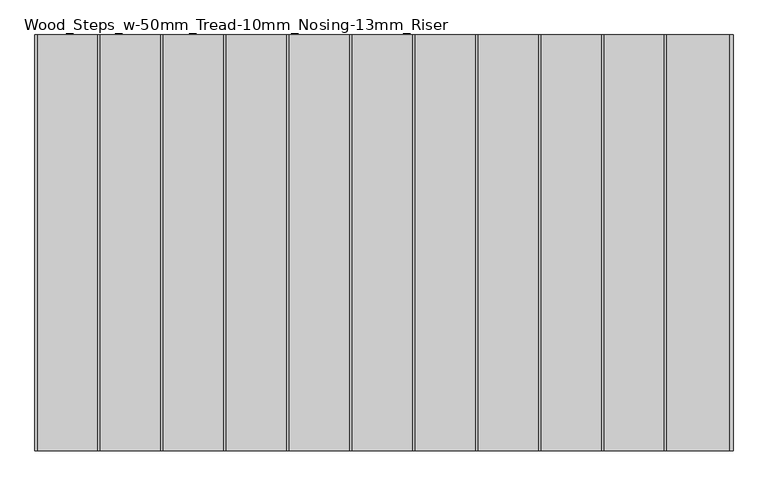
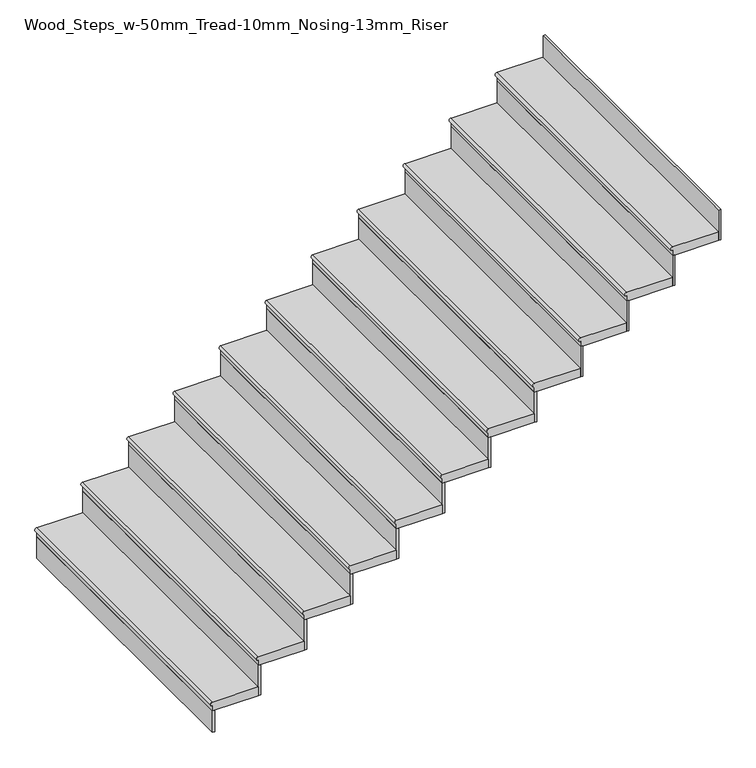
"""IFC4 building model written with IfcOpenShell, lengths in millimetres: stair flight geometry, Wood_Steps_w-50mm_Tread-10mm_Nosing-13mm_Riser."""

from ifc_helpers import new_model, si_unit, frame, origin, place, context, project, spatial, circle_curve, faceted_brep, source, transform, mapped, element, save
from ifc_brep_helpers import plane_surface, cylinder_surface, advanced_brep


def wood_steps_w_50mm_tread_10mm_nosing_13mm_riser_0f893a5b(model_context):
    return source(origin(), model_context, "Body", "SolidModel", [
        advanced_brep(
        [(-512.9988863, -6137.6352742, 153.9130435), (-512.9988863, -6137.6352742, 173.9130435), (-512.9988863, -4486.6352742, 173.9130435), (-512.9988863, -4486.6352742, 153.9130435), (-262.9988863, -4486.6352742, 173.9130435), (-262.9988863, -6137.6352742, 173.9130435), (-512.9988863, -4486.6352742, 123.9130435), (-262.9988863, -4486.6352742, 123.9130435), (-262.9988863, -6137.6352742, 123.9130435), (-512.9988863, -6137.6352742, 123.9130435)],
        [
            (0, 1, circle_curve(frame((-512.9988863, -6137.6352742, 163.9130435), z_axis=(0.0, 1.0, 0.0), x_axis=(1.0, 0.0, 0.0)), 10.0)),
            (1, 2),
            (2, 3, circle_curve(frame((-512.9988863, -4486.6352742, 163.9130435), z_axis=(0.0, -1.0, 0.0), x_axis=(1.0, 0.0, 0.0)), 10.0)),
            (3, 0),
            (4, 2),
            (1, 5),
            (5, 4),
            (6, 7),
            (7, 8),
            (8, 9),
            (9, 6),
            (4, 7),
            (6, 3),
            (9, 0),
            (8, 5),
        ],
        [
            cylinder_surface(frame((-512.9988863, -6137.6352742, 163.9130435), z_axis=(0.0, -1.0, 0.0), x_axis=(1.0, 0.0, 0.0)), 10.0),
            plane_surface(frame((-522.9988863, -4486.6352742, 173.9130435), z_axis=(0.0, 0.0, 1.0), x_axis=(-1.0, 0.0, 0.0))),
            plane_surface(frame((-522.9988863, -4486.6352742, 123.9130435), z_axis=(0.0, 0.0, -1.0), x_axis=(1.0, 0.0, 0.0))),
            plane_surface(frame((-262.9988863, -4486.6352742, 173.9130435), z_axis=(0.0, 1.0, 0.0), x_axis=(0.0, 0.0, -1.0))),
            plane_surface(frame((-512.9988863, -4486.6352742, 173.9130435), z_axis=(-1.0, 0.0, 0.0), x_axis=(0.0, 0.0, -1.0))),
            plane_surface(frame((-512.9988863, -6137.6352742, 173.9130435), z_axis=(0.0, -1.0, 0.0), x_axis=(0.0, 0.0, -1.0))),
            plane_surface(frame((-262.9988863, -6137.6352742, 173.9130435), z_axis=(1.0, 0.0, 0.0), x_axis=(0.0, 0.0, -1.0))),
        ],
        [
            (0, [[1, 2, 3, 4]]),
            (1, [[5, -2, 6, 7]]),
            (2, [[8, 9, 10, 11]]),
            (3, [[-5, 12, -8, 13, -3]]),
            (4, [[-11, 14, -4, -13]]),
            (5, [[-6, -1, -14, -10, 15]]),
            (6, [[-7, -15, -9, -12]]),
        ],
    ),
        faceted_brep([(-512.9988863, -6137.6352742, 123.9130435), (-512.9988863, -6137.6352742, 0.0), (-500.4988863, -6137.6352742, 0.0), (-500.4988863, -6137.6352742, 123.9130435), (-512.9988863, -4486.6352742, 123.9130435), (-500.4988863, -4486.6352742, 123.9130435), (-500.4988863, -4486.6352742, 0.0), (-512.9988863, -4486.6352742, 0.0)], [[[0, 1, 2, 3]], [[4, 5, 6, 7]], [[1, 0, 4, 7]], [[2, 1, 7, 6]], [[3, 2, 6, 5]], [[0, 3, 5, 4]]]),
        faceted_brep([(-262.9988863, -6137.6352742, 297.826087), (-262.9988863, -6137.6352742, 123.9130435), (-250.4988863, -6137.6352742, 123.9130435), (-250.4988863, -6137.6352742, 297.826087), (-262.9988863, -4486.6352742, 297.826087), (-250.4988863, -4486.6352742, 297.826087), (-250.4988863, -4486.6352742, 123.9130435), (-262.9988863, -4486.6352742, 123.9130435)], [[[0, 1, 2, 3]], [[4, 5, 6, 7]], [[1, 0, 4, 7]], [[2, 1, 7, 6]], [[3, 2, 6, 5]], [[0, 3, 5, 4]]]),
        advanced_brep(
        [(-12.9988863, -4486.6352742, 347.826087), (-262.9988863, -4486.6352742, 347.826087), (-262.9988863, -6137.6352742, 347.826087), (-12.9988863, -6137.6352742, 347.826087), (-262.9988863, -4486.6352742, 297.826087), (-12.9988863, -4486.6352742, 297.826087), (-12.9988863, -6137.6352742, 297.826087), (-262.9988863, -6137.6352742, 297.826087), (-262.9988863, -4486.6352742, 327.826087), (-262.9988863, -6137.6352742, 327.826087)],
        [
            (0, 1),
            (1, 2),
            (2, 3),
            (3, 0),
            (4, 5),
            (5, 6),
            (6, 7),
            (7, 4),
            (0, 5),
            (4, 8),
            (8, 1, circle_curve(frame((-262.9988863, -4486.6352742, 337.826087), z_axis=(0.0, 1.0, 0.0), x_axis=(1.0, 0.0, 0.0)), 10.0)),
            (7, 9),
            (9, 8),
            (2, 9, circle_curve(frame((-262.9988863, -6137.6352742, 337.826087), z_axis=(0.0, -1.0, 0.0), x_axis=(1.0, 0.0, 0.0)), 10.0)),
            (6, 3),
        ],
        [
            plane_surface(frame((-522.9988863, -4486.6352742, 347.826087), z_axis=(0.0, 0.0, 1.0), x_axis=(-1.0, 0.0, 0.0))),
            plane_surface(frame((-522.9988863, -4486.6352742, 297.826087), z_axis=(0.0, 0.0, -1.0), x_axis=(1.0, 0.0, 0.0))),
            plane_surface(frame((-12.9988863, -4486.6352742, 347.826087), z_axis=(0.0, 1.0, 0.0), x_axis=(0.0, 0.0, -1.0))),
            plane_surface(frame((-262.9988863, -4486.6352742, 347.826087), z_axis=(-1.0, 0.0, 0.0), x_axis=(0.0, 0.0, -1.0))),
            plane_surface(frame((-262.9988863, -6137.6352742, 347.826087), z_axis=(0.0, -1.0, 0.0), x_axis=(0.0, 0.0, -1.0))),
            plane_surface(frame((-12.9988863, -6137.6352742, 347.826087), z_axis=(1.0, 0.0, 0.0), x_axis=(0.0, 0.0, -1.0))),
            cylinder_surface(frame((-262.9988863, -6137.6352742, 337.826087), z_axis=(0.0, -1.0, 0.0), x_axis=(1.0, 0.0, 0.0)), 10.0),
        ],
        [
            (0, [[1, 2, 3, 4]]),
            (1, [[5, 6, 7, 8]]),
            (2, [[-1, 9, -5, 10, 11]]),
            (3, [[-8, 12, 13, -10]]),
            (4, [[-3, 14, -12, -7, 15]]),
            (5, [[-4, -15, -6, -9]]),
            (6, [[-14, -2, -11, -13]]),
        ],
    ),
        faceted_brep([(-12.9988863, -6137.6352742, 471.7391304), (-12.9988863, -6137.6352742, 297.826087), (-0.4988863, -6137.6352742, 297.826087), (-0.4988863, -6137.6352742, 471.7391304), (-12.9988863, -4486.6352742, 471.7391304), (-0.4988863, -4486.6352742, 471.7391304), (-0.4988863, -4486.6352742, 297.826087), (-12.9988863, -4486.6352742, 297.826087)], [[[0, 1, 2, 3]], [[4, 5, 6, 7]], [[1, 0, 4, 7]], [[2, 1, 7, 6]], [[3, 2, 6, 5]], [[0, 3, 5, 4]]]),
        advanced_brep(
        [(237.0011137, -4486.6352742, 521.7391304), (-12.9988863, -4486.6352742, 521.7391304), (-12.9988863, -6137.6352742, 521.7391304), (237.0011137, -6137.6352742, 521.7391304), (-12.9988863, -4486.6352742, 471.7391304), (237.0011137, -4486.6352742, 471.7391304), (237.0011137, -6137.6352742, 471.7391304), (-12.9988863, -6137.6352742, 471.7391304), (-12.9988863, -4486.6352742, 501.7391304), (-12.9988863, -6137.6352742, 501.7391304)],
        [
            (0, 1),
            (1, 2),
            (2, 3),
            (3, 0),
            (4, 5),
            (5, 6),
            (6, 7),
            (7, 4),
            (0, 5),
            (4, 8),
            (8, 1, circle_curve(frame((-12.9988863, -4486.6352742, 511.7391304), z_axis=(0.0, 1.0, 0.0), x_axis=(1.0, 0.0, 0.0)), 10.0)),
            (7, 9),
            (9, 8),
            (2, 9, circle_curve(frame((-12.9988863, -6137.6352742, 511.7391304), z_axis=(0.0, -1.0, 0.0), x_axis=(1.0, 0.0, 0.0)), 10.0)),
            (6, 3),
        ],
        [
            plane_surface(frame((-272.9988863, -4486.6352742, 521.7391304), z_axis=(0.0, 0.0, 1.0), x_axis=(-1.0, 0.0, 0.0))),
            plane_surface(frame((-272.9988863, -4486.6352742, 471.7391304), z_axis=(0.0, 0.0, -1.0), x_axis=(1.0, 0.0, 0.0))),
            plane_surface(frame((237.0011137, -4486.6352742, 521.7391304), z_axis=(0.0, 1.0, 0.0), x_axis=(0.0, 0.0, -1.0))),
            plane_surface(frame((-12.9988863, -4486.6352742, 521.7391304), z_axis=(-1.0, 0.0, 0.0), x_axis=(0.0, 0.0, -1.0))),
            plane_surface(frame((-12.9988863, -6137.6352742, 521.7391304), z_axis=(0.0, -1.0, 0.0), x_axis=(0.0, 0.0, -1.0))),
            plane_surface(frame((237.0011137, -6137.6352742, 521.7391304), z_axis=(1.0, 0.0, 0.0), x_axis=(0.0, 0.0, -1.0))),
            cylinder_surface(frame((-12.9988863, -6137.6352742, 511.7391304), z_axis=(0.0, -1.0, 0.0), x_axis=(1.0, 0.0, 0.0)), 10.0),
        ],
        [
            (0, [[1, 2, 3, 4]]),
            (1, [[5, 6, 7, 8]]),
            (2, [[-1, 9, -5, 10, 11]]),
            (3, [[-8, 12, 13, -10]]),
            (4, [[-3, 14, -12, -7, 15]]),
            (5, [[-4, -15, -6, -9]]),
            (6, [[-14, -2, -11, -13]]),
        ],
    ),
        faceted_brep([(237.0011137, -6137.6352742, 645.6521739), (237.0011137, -6137.6352742, 471.7391304), (249.5011137, -6137.6352742, 471.7391304), (249.5011137, -6137.6352742, 645.6521739), (237.0011137, -4486.6352742, 645.6521739), (249.5011137, -4486.6352742, 645.6521739), (249.5011137, -4486.6352742, 471.7391304), (237.0011137, -4486.6352742, 471.7391304)], [[[0, 1, 2, 3]], [[4, 5, 6, 7]], [[1, 0, 4, 7]], [[2, 1, 7, 6]], [[3, 2, 6, 5]], [[0, 3, 5, 4]]]),
        advanced_brep(
        [(487.0011137, -4486.6352742, 695.6521739), (237.0011137, -4486.6352742, 695.6521739), (237.0011137, -6137.6352742, 695.6521739), (487.0011137, -6137.6352742, 695.6521739), (237.0011137, -4486.6352742, 645.6521739), (487.0011137, -4486.6352742, 645.6521739), (487.0011137, -6137.6352742, 645.6521739), (237.0011137, -6137.6352742, 645.6521739), (237.0011137, -4486.6352742, 675.6521739), (237.0011137, -6137.6352742, 675.6521739)],
        [
            (0, 1),
            (1, 2),
            (2, 3),
            (3, 0),
            (4, 5),
            (5, 6),
            (6, 7),
            (7, 4),
            (0, 5),
            (4, 8),
            (8, 1, circle_curve(frame((237.0011137, -4486.6352742, 685.6521739), z_axis=(0.0, 1.0, 0.0), x_axis=(1.0, 0.0, 0.0)), 10.0)),
            (7, 9),
            (9, 8),
            (2, 9, circle_curve(frame((237.0011137, -6137.6352742, 685.6521739), z_axis=(0.0, -1.0, 0.0), x_axis=(1.0, 0.0, 0.0)), 10.0)),
            (6, 3),
        ],
        [
            plane_surface(frame((-22.9988863, -4486.6352742, 695.6521739), z_axis=(0.0, 0.0, 1.0), x_axis=(-1.0, 0.0, 0.0))),
            plane_surface(frame((-22.9988863, -4486.6352742, 645.6521739), z_axis=(0.0, 0.0, -1.0), x_axis=(1.0, 0.0, 0.0))),
            plane_surface(frame((487.0011137, -4486.6352742, 695.6521739), z_axis=(0.0, 1.0, 0.0), x_axis=(0.0, 0.0, -1.0))),
            plane_surface(frame((237.0011137, -4486.6352742, 695.6521739), z_axis=(-1.0, 0.0, 0.0), x_axis=(0.0, 0.0, -1.0))),
            plane_surface(frame((237.0011137, -6137.6352742, 695.6521739), z_axis=(0.0, -1.0, 0.0), x_axis=(0.0, 0.0, -1.0))),
            plane_surface(frame((487.0011137, -6137.6352742, 695.6521739), z_axis=(1.0, 0.0, 0.0), x_axis=(0.0, 0.0, -1.0))),
            cylinder_surface(frame((237.0011137, -6137.6352742, 685.6521739), z_axis=(0.0, -1.0, 0.0), x_axis=(1.0, 0.0, 0.0)), 10.0),
        ],
        [
            (0, [[1, 2, 3, 4]]),
            (1, [[5, 6, 7, 8]]),
            (2, [[-1, 9, -5, 10, 11]]),
            (3, [[-8, 12, 13, -10]]),
            (4, [[-3, 14, -12, -7, 15]]),
            (5, [[-4, -15, -6, -9]]),
            (6, [[-14, -2, -11, -13]]),
        ],
    ),
        faceted_brep([(487.0011137, -6137.6352742, 819.5652174), (487.0011137, -6137.6352742, 645.6521739), (499.5011137, -6137.6352742, 645.6521739), (499.5011137, -6137.6352742, 819.5652174), (487.0011137, -4486.6352742, 819.5652174), (499.5011137, -4486.6352742, 819.5652174), (499.5011137, -4486.6352742, 645.6521739), (487.0011137, -4486.6352742, 645.6521739)], [[[0, 1, 2, 3]], [[4, 5, 6, 7]], [[1, 0, 4, 7]], [[2, 1, 7, 6]], [[3, 2, 6, 5]], [[0, 3, 5, 4]]]),
        advanced_brep(
        [(737.0011137, -4486.6352742, 869.5652174), (487.0011137, -4486.6352742, 869.5652174), (487.0011137, -6137.6352742, 869.5652174), (737.0011137, -6137.6352742, 869.5652174), (487.0011137, -4486.6352742, 819.5652174), (737.0011137, -4486.6352742, 819.5652174), (737.0011137, -6137.6352742, 819.5652174), (487.0011137, -6137.6352742, 819.5652174), (487.0011137, -4486.6352742, 849.5652174), (487.0011137, -6137.6352742, 849.5652174)],
        [
            (0, 1),
            (1, 2),
            (2, 3),
            (3, 0),
            (4, 5),
            (5, 6),
            (6, 7),
            (7, 4),
            (0, 5),
            (4, 8),
            (8, 1, circle_curve(frame((487.0011137, -4486.6352742, 859.5652174), z_axis=(0.0, 1.0, 0.0), x_axis=(1.0, 0.0, 0.0)), 10.0)),
            (7, 9),
            (9, 8),
            (2, 9, circle_curve(frame((487.0011137, -6137.6352742, 859.5652174), z_axis=(0.0, -1.0, 0.0), x_axis=(1.0, 0.0, 0.0)), 10.0)),
            (6, 3),
        ],
        [
            plane_surface(frame((227.0011137, -4486.6352742, 869.5652174), z_axis=(0.0, 0.0, 1.0), x_axis=(-1.0, 0.0, 0.0))),
            plane_surface(frame((227.0011137, -4486.6352742, 819.5652174), z_axis=(0.0, 0.0, -1.0), x_axis=(1.0, 0.0, 0.0))),
            plane_surface(frame((737.0011137, -4486.6352742, 869.5652174), z_axis=(0.0, 1.0, 0.0), x_axis=(0.0, 0.0, -1.0))),
            plane_surface(frame((487.0011137, -4486.6352742, 869.5652174), z_axis=(-1.0, 0.0, 0.0), x_axis=(0.0, 0.0, -1.0))),
            plane_surface(frame((487.0011137, -6137.6352742, 869.5652174), z_axis=(0.0, -1.0, 0.0), x_axis=(0.0, 0.0, -1.0))),
            plane_surface(frame((737.0011137, -6137.6352742, 869.5652174), z_axis=(1.0, 0.0, 0.0), x_axis=(0.0, 0.0, -1.0))),
            cylinder_surface(frame((487.0011137, -6137.6352742, 859.5652174), z_axis=(0.0, -1.0, 0.0), x_axis=(1.0, 0.0, 0.0)), 10.0),
        ],
        [
            (0, [[1, 2, 3, 4]]),
            (1, [[5, 6, 7, 8]]),
            (2, [[-1, 9, -5, 10, 11]]),
            (3, [[-8, 12, 13, -10]]),
            (4, [[-3, 14, -12, -7, 15]]),
            (5, [[-4, -15, -6, -9]]),
            (6, [[-14, -2, -11, -13]]),
        ],
    ),
        faceted_brep([(737.0011137, -6137.6352742, 993.4782609), (737.0011137, -6137.6352742, 819.5652174), (749.5011137, -6137.6352742, 819.5652174), (749.5011137, -6137.6352742, 993.4782609), (737.0011137, -4486.6352742, 993.4782609), (749.5011137, -4486.6352742, 993.4782609), (749.5011137, -4486.6352742, 819.5652174), (737.0011137, -4486.6352742, 819.5652174)], [[[0, 1, 2, 3]], [[4, 5, 6, 7]], [[1, 0, 4, 7]], [[2, 1, 7, 6]], [[3, 2, 6, 5]], [[0, 3, 5, 4]]]),
        advanced_brep(
        [(987.0011137, -4486.6352742, 1043.4782609), (737.0011137, -4486.6352742, 1043.4782609), (737.0011137, -6137.6352742, 1043.4782609), (987.0011137, -6137.6352742, 1043.4782609), (737.0011137, -4486.6352742, 993.4782609), (987.0011137, -4486.6352742, 993.4782609), (987.0011137, -6137.6352742, 993.4782609), (737.0011137, -6137.6352742, 993.4782609), (737.0011137, -4486.6352742, 1023.4782609), (737.0011137, -6137.6352742, 1023.4782609)],
        [
            (0, 1),
            (1, 2),
            (2, 3),
            (3, 0),
            (4, 5),
            (5, 6),
            (6, 7),
            (7, 4),
            (0, 5),
            (4, 8),
            (8, 1, circle_curve(frame((737.0011137, -4486.6352742, 1033.4782609), z_axis=(0.0, 1.0, 0.0), x_axis=(1.0, 0.0, 0.0)), 10.0)),
            (7, 9),
            (9, 8),
            (2, 9, circle_curve(frame((737.0011137, -6137.6352742, 1033.4782609), z_axis=(0.0, -1.0, 0.0), x_axis=(1.0, 0.0, 0.0)), 10.0)),
            (6, 3),
        ],
        [
            plane_surface(frame((477.0011137, -4486.6352742, 1043.4782609), z_axis=(0.0, 0.0, 1.0), x_axis=(-1.0, 0.0, 0.0))),
            plane_surface(frame((477.0011137, -4486.6352742, 993.4782609), z_axis=(0.0, 0.0, -1.0), x_axis=(1.0, 0.0, 0.0))),
            plane_surface(frame((987.0011137, -4486.6352742, 1043.4782609), z_axis=(0.0, 1.0, 0.0), x_axis=(0.0, 0.0, -1.0))),
            plane_surface(frame((737.0011137, -4486.6352742, 1043.4782609), z_axis=(-1.0, 0.0, 0.0), x_axis=(0.0, 0.0, -1.0))),
            plane_surface(frame((737.0011137, -6137.6352742, 1043.4782609), z_axis=(0.0, -1.0, 0.0), x_axis=(0.0, 0.0, -1.0))),
            plane_surface(frame((987.0011137, -6137.6352742, 1043.4782609), z_axis=(1.0, 0.0, 0.0), x_axis=(0.0, 0.0, -1.0))),
            cylinder_surface(frame((737.0011137, -6137.6352742, 1033.4782609), z_axis=(0.0, -1.0, 0.0), x_axis=(1.0, 0.0, 0.0)), 10.0),
        ],
        [
            (0, [[1, 2, 3, 4]]),
            (1, [[5, 6, 7, 8]]),
            (2, [[-1, 9, -5, 10, 11]]),
            (3, [[-8, 12, 13, -10]]),
            (4, [[-3, 14, -12, -7, 15]]),
            (5, [[-4, -15, -6, -9]]),
            (6, [[-14, -2, -11, -13]]),
        ],
    ),
        faceted_brep([(987.0011137, -6137.6352742, 1167.3913043), (987.0011137, -6137.6352742, 993.4782609), (999.5011137, -6137.6352742, 993.4782609), (999.5011137, -6137.6352742, 1167.3913043), (987.0011137, -4486.6352742, 1167.3913043), (999.5011137, -4486.6352742, 1167.3913043), (999.5011137, -4486.6352742, 993.4782609), (987.0011137, -4486.6352742, 993.4782609)], [[[0, 1, 2, 3]], [[4, 5, 6, 7]], [[1, 0, 4, 7]], [[2, 1, 7, 6]], [[3, 2, 6, 5]], [[0, 3, 5, 4]]]),
        advanced_brep(
        [(1237.0011137, -4486.6352742, 1217.3913043), (987.0011137, -4486.6352742, 1217.3913043), (987.0011137, -6137.6352742, 1217.3913043), (1237.0011137, -6137.6352742, 1217.3913043), (987.0011137, -4486.6352742, 1167.3913043), (1237.0011137, -4486.6352742, 1167.3913043), (1237.0011137, -6137.6352742, 1167.3913043), (987.0011137, -6137.6352742, 1167.3913043), (987.0011137, -4486.6352742, 1197.3913043), (987.0011137, -6137.6352742, 1197.3913043)],
        [
            (0, 1),
            (1, 2),
            (2, 3),
            (3, 0),
            (4, 5),
            (5, 6),
            (6, 7),
            (7, 4),
            (0, 5),
            (4, 8),
            (8, 1, circle_curve(frame((987.0011137, -4486.6352742, 1207.3913043), z_axis=(0.0, 1.0, 0.0), x_axis=(1.0, 0.0, 0.0)), 10.0)),
            (7, 9),
            (9, 8),
            (2, 9, circle_curve(frame((987.0011137, -6137.6352742, 1207.3913043), z_axis=(0.0, -1.0, 0.0), x_axis=(1.0, 0.0, 0.0)), 10.0)),
            (6, 3),
        ],
        [
            plane_surface(frame((727.0011137, -4486.6352742, 1217.3913043), z_axis=(0.0, 0.0, 1.0), x_axis=(-1.0, 0.0, 0.0))),
            plane_surface(frame((727.0011137, -4486.6352742, 1167.3913043), z_axis=(0.0, 0.0, -1.0), x_axis=(1.0, 0.0, 0.0))),
            plane_surface(frame((1237.0011137, -4486.6352742, 1217.3913043), z_axis=(0.0, 1.0, 0.0), x_axis=(0.0, 0.0, -1.0))),
            plane_surface(frame((987.0011137, -4486.6352742, 1217.3913043), z_axis=(-1.0, 0.0, 0.0), x_axis=(0.0, 0.0, -1.0))),
            plane_surface(frame((987.0011137, -6137.6352742, 1217.3913043), z_axis=(0.0, -1.0, 0.0), x_axis=(0.0, 0.0, -1.0))),
            plane_surface(frame((1237.0011137, -6137.6352742, 1217.3913043), z_axis=(1.0, 0.0, 0.0), x_axis=(0.0, 0.0, -1.0))),
            cylinder_surface(frame((987.0011137, -6137.6352742, 1207.3913043), z_axis=(0.0, -1.0, 0.0), x_axis=(1.0, 0.0, 0.0)), 10.0),
        ],
        [
            (0, [[1, 2, 3, 4]]),
            (1, [[5, 6, 7, 8]]),
            (2, [[-1, 9, -5, 10, 11]]),
            (3, [[-8, 12, 13, -10]]),
            (4, [[-3, 14, -12, -7, 15]]),
            (5, [[-4, -15, -6, -9]]),
            (6, [[-14, -2, -11, -13]]),
        ],
    ),
        faceted_brep([(1237.0011137, -6137.6352742, 1341.3043478), (1237.0011137, -6137.6352742, 1167.3913043), (1249.5011137, -6137.6352742, 1167.3913043), (1249.5011137, -6137.6352742, 1341.3043478), (1237.0011137, -4486.6352742, 1341.3043478), (1249.5011137, -4486.6352742, 1341.3043478), (1249.5011137, -4486.6352742, 1167.3913043), (1237.0011137, -4486.6352742, 1167.3913043)], [[[0, 1, 2, 3]], [[4, 5, 6, 7]], [[1, 0, 4, 7]], [[2, 1, 7, 6]], [[3, 2, 6, 5]], [[0, 3, 5, 4]]]),
        advanced_brep(
        [(1487.0011137, -4486.6352742, 1391.3043478), (1237.0011137, -4486.6352742, 1391.3043478), (1237.0011137, -6137.6352742, 1391.3043478), (1487.0011137, -6137.6352742, 1391.3043478), (1237.0011137, -4486.6352742, 1341.3043478), (1487.0011137, -4486.6352742, 1341.3043478), (1487.0011137, -6137.6352742, 1341.3043478), (1237.0011137, -6137.6352742, 1341.3043478), (1237.0011137, -4486.6352742, 1371.3043478), (1237.0011137, -6137.6352742, 1371.3043478)],
        [
            (0, 1),
            (1, 2),
            (2, 3),
            (3, 0),
            (4, 5),
            (5, 6),
            (6, 7),
            (7, 4),
            (0, 5),
            (4, 8),
            (8, 1, circle_curve(frame((1237.0011137, -4486.6352742, 1381.3043478), z_axis=(0.0, 1.0, 0.0), x_axis=(1.0, 0.0, 0.0)), 10.0)),
            (7, 9),
            (9, 8),
            (2, 9, circle_curve(frame((1237.0011137, -6137.6352742, 1381.3043478), z_axis=(0.0, -1.0, 0.0), x_axis=(1.0, 0.0, 0.0)), 10.0)),
            (6, 3),
        ],
        [
            plane_surface(frame((977.0011137, -4486.6352742, 1391.3043478), z_axis=(0.0, 0.0, 1.0), x_axis=(-1.0, 0.0, 0.0))),
            plane_surface(frame((977.0011137, -4486.6352742, 1341.3043478), z_axis=(0.0, 0.0, -1.0), x_axis=(1.0, 0.0, 0.0))),
            plane_surface(frame((1487.0011137, -4486.6352742, 1391.3043478), z_axis=(0.0, 1.0, 0.0), x_axis=(0.0, 0.0, -1.0))),
            plane_surface(frame((1237.0011137, -4486.6352742, 1391.3043478), z_axis=(-1.0, 0.0, 0.0), x_axis=(0.0, 0.0, -1.0))),
            plane_surface(frame((1237.0011137, -6137.6352742, 1391.3043478), z_axis=(0.0, -1.0, 0.0), x_axis=(0.0, 0.0, -1.0))),
            plane_surface(frame((1487.0011137, -6137.6352742, 1391.3043478), z_axis=(1.0, 0.0, 0.0), x_axis=(0.0, 0.0, -1.0))),
            cylinder_surface(frame((1237.0011137, -6137.6352742, 1381.3043478), z_axis=(0.0, -1.0, 0.0), x_axis=(1.0, 0.0, 0.0)), 10.0),
        ],
        [
            (0, [[1, 2, 3, 4]]),
            (1, [[5, 6, 7, 8]]),
            (2, [[-1, 9, -5, 10, 11]]),
            (3, [[-8, 12, 13, -10]]),
            (4, [[-3, 14, -12, -7, 15]]),
            (5, [[-4, -15, -6, -9]]),
            (6, [[-14, -2, -11, -13]]),
        ],
    ),
        faceted_brep([(1487.0011137, -6137.6352742, 1515.2173913), (1487.0011137, -6137.6352742, 1341.3043478), (1499.5011137, -6137.6352742, 1341.3043478), (1499.5011137, -6137.6352742, 1515.2173913), (1487.0011137, -4486.6352742, 1515.2173913), (1499.5011137, -4486.6352742, 1515.2173913), (1499.5011137, -4486.6352742, 1341.3043478), (1487.0011137, -4486.6352742, 1341.3043478)], [[[0, 1, 2, 3]], [[4, 5, 6, 7]], [[1, 0, 4, 7]], [[2, 1, 7, 6]], [[3, 2, 6, 5]], [[0, 3, 5, 4]]]),
        advanced_brep(
        [(1737.0011137, -4486.6352742, 1565.2173913), (1487.0011137, -4486.6352742, 1565.2173913), (1487.0011137, -6137.6352742, 1565.2173913), (1737.0011137, -6137.6352742, 1565.2173913), (1487.0011137, -4486.6352742, 1515.2173913), (1737.0011137, -4486.6352742, 1515.2173913), (1737.0011137, -6137.6352742, 1515.2173913), (1487.0011137, -6137.6352742, 1515.2173913), (1487.0011137, -4486.6352742, 1545.2173913), (1487.0011137, -6137.6352742, 1545.2173913)],
        [
            (0, 1),
            (1, 2),
            (2, 3),
            (3, 0),
            (4, 5),
            (5, 6),
            (6, 7),
            (7, 4),
            (0, 5),
            (4, 8),
            (8, 1, circle_curve(frame((1487.0011137, -4486.6352742, 1555.2173913), z_axis=(0.0, 1.0, 0.0), x_axis=(1.0, 0.0, 0.0)), 10.0)),
            (7, 9),
            (9, 8),
            (2, 9, circle_curve(frame((1487.0011137, -6137.6352742, 1555.2173913), z_axis=(0.0, -1.0, 0.0), x_axis=(1.0, 0.0, 0.0)), 10.0)),
            (6, 3),
        ],
        [
            plane_surface(frame((1227.0011137, -4486.6352742, 1565.2173913), z_axis=(0.0, 0.0, 1.0), x_axis=(-1.0, 0.0, 0.0))),
            plane_surface(frame((1227.0011137, -4486.6352742, 1515.2173913), z_axis=(0.0, 0.0, -1.0), x_axis=(1.0, 0.0, 0.0))),
            plane_surface(frame((1737.0011137, -4486.6352742, 1565.2173913), z_axis=(0.0, 1.0, 0.0), x_axis=(0.0, 0.0, -1.0))),
            plane_surface(frame((1487.0011137, -4486.6352742, 1565.2173913), z_axis=(-1.0, 0.0, 0.0), x_axis=(0.0, 0.0, -1.0))),
            plane_surface(frame((1487.0011137, -6137.6352742, 1565.2173913), z_axis=(0.0, -1.0, 0.0), x_axis=(0.0, 0.0, -1.0))),
            plane_surface(frame((1737.0011137, -6137.6352742, 1565.2173913), z_axis=(1.0, 0.0, 0.0), x_axis=(0.0, 0.0, -1.0))),
            cylinder_surface(frame((1487.0011137, -6137.6352742, 1555.2173913), z_axis=(0.0, -1.0, 0.0), x_axis=(1.0, 0.0, 0.0)), 10.0),
        ],
        [
            (0, [[1, 2, 3, 4]]),
            (1, [[5, 6, 7, 8]]),
            (2, [[-1, 9, -5, 10, 11]]),
            (3, [[-8, 12, 13, -10]]),
            (4, [[-3, 14, -12, -7, 15]]),
            (5, [[-4, -15, -6, -9]]),
            (6, [[-14, -2, -11, -13]]),
        ],
    ),
        faceted_brep([(1737.0011137, -6137.6352742, 1689.1304348), (1737.0011137, -6137.6352742, 1515.2173913), (1749.5011137, -6137.6352742, 1515.2173913), (1749.5011137, -6137.6352742, 1689.1304348), (1737.0011137, -4486.6352742, 1689.1304348), (1749.5011137, -4486.6352742, 1689.1304348), (1749.5011137, -4486.6352742, 1515.2173913), (1737.0011137, -4486.6352742, 1515.2173913)], [[[0, 1, 2, 3]], [[4, 5, 6, 7]], [[1, 0, 4, 7]], [[2, 1, 7, 6]], [[3, 2, 6, 5]], [[0, 3, 5, 4]]]),
        advanced_brep(
        [(1987.0011137, -4486.6352742, 1739.1304348), (1737.0011137, -4486.6352742, 1739.1304348), (1737.0011137, -6137.6352742, 1739.1304348), (1987.0011137, -6137.6352742, 1739.1304348), (1737.0011137, -4486.6352742, 1689.1304348), (1987.0011137, -4486.6352742, 1689.1304348), (1987.0011137, -6137.6352742, 1689.1304348), (1737.0011137, -6137.6352742, 1689.1304348), (1737.0011137, -4486.6352742, 1719.1304348), (1737.0011137, -6137.6352742, 1719.1304348)],
        [
            (0, 1),
            (1, 2),
            (2, 3),
            (3, 0),
            (4, 5),
            (5, 6),
            (6, 7),
            (7, 4),
            (0, 5),
            (4, 8),
            (8, 1, circle_curve(frame((1737.0011137, -4486.6352742, 1729.1304348), z_axis=(0.0, 1.0, 0.0), x_axis=(1.0, 0.0, 0.0)), 10.0)),
            (7, 9),
            (9, 8),
            (2, 9, circle_curve(frame((1737.0011137, -6137.6352742, 1729.1304348), z_axis=(0.0, -1.0, 0.0), x_axis=(1.0, 0.0, 0.0)), 10.0)),
            (6, 3),
        ],
        [
            plane_surface(frame((1477.0011137, -4486.6352742, 1739.1304348), z_axis=(0.0, 0.0, 1.0), x_axis=(-1.0, 0.0, 0.0))),
            plane_surface(frame((1477.0011137, -4486.6352742, 1689.1304348), z_axis=(0.0, 0.0, -1.0), x_axis=(1.0, 0.0, 0.0))),
            plane_surface(frame((1987.0011137, -4486.6352742, 1739.1304348), z_axis=(0.0, 1.0, 0.0), x_axis=(0.0, 0.0, -1.0))),
            plane_surface(frame((1737.0011137, -4486.6352742, 1739.1304348), z_axis=(-1.0, 0.0, 0.0), x_axis=(0.0, 0.0, -1.0))),
            plane_surface(frame((1737.0011137, -6137.6352742, 1739.1304348), z_axis=(0.0, -1.0, 0.0), x_axis=(0.0, 0.0, -1.0))),
            plane_surface(frame((1987.0011137, -6137.6352742, 1739.1304348), z_axis=(1.0, 0.0, 0.0), x_axis=(0.0, 0.0, -1.0))),
            cylinder_surface(frame((1737.0011137, -6137.6352742, 1729.1304348), z_axis=(0.0, -1.0, 0.0), x_axis=(1.0, 0.0, 0.0)), 10.0),
        ],
        [
            (0, [[1, 2, 3, 4]]),
            (1, [[5, 6, 7, 8]]),
            (2, [[-1, 9, -5, 10, 11]]),
            (3, [[-8, 12, 13, -10]]),
            (4, [[-3, 14, -12, -7, 15]]),
            (5, [[-4, -15, -6, -9]]),
            (6, [[-14, -2, -11, -13]]),
        ],
    ),
        faceted_brep([(2237.0011137, -6137.6352742, 2036.9565217), (2237.0011137, -6137.6352742, 1863.0434783), (2249.5011137, -6137.6352742, 1863.0434783), (2249.5011137, -6137.6352742, 2036.9565217), (2237.0011137, -4486.6352742, 2036.9565217), (2249.5011137, -4486.6352742, 2036.9565217), (2249.5011137, -4486.6352742, 1863.0434783), (2237.0011137, -4486.6352742, 1863.0434783)], [[[0, 1, 2, 3]], [[4, 5, 6, 7]], [[1, 0, 4, 7]], [[2, 1, 7, 6]], [[3, 2, 6, 5]], [[0, 3, 5, 4]]]),
        faceted_brep([(1987.0011137, -6137.6352742, 1863.0434783), (1987.0011137, -6137.6352742, 1689.1304348), (1999.5011137, -6137.6352742, 1689.1304348), (1999.5011137, -6137.6352742, 1863.0434783), (1987.0011137, -4486.6352742, 1863.0434783), (1999.5011137, -4486.6352742, 1863.0434783), (1999.5011137, -4486.6352742, 1689.1304348), (1987.0011137, -4486.6352742, 1689.1304348)], [[[0, 1, 2, 3]], [[4, 5, 6, 7]], [[1, 0, 4, 7]], [[2, 1, 7, 6]], [[3, 2, 6, 5]], [[0, 3, 5, 4]]]),
        advanced_brep(
        [(2237.0011137, -4486.6352742, 1913.0434783), (2227.0011137, -4486.6352742, 1913.0434783), (1987.0011137, -4486.6352742, 1913.0434783), (1987.0011137, -6137.6352742, 1913.0434783), (2237.0011137, -6137.6352742, 1913.0434783), (2227.0011137, -4486.6352742, 1863.0434783), (2237.0011137, -4486.6352742, 1863.0434783), (2237.0011137, -6137.6352742, 1863.0434783), (1987.0011137, -6137.6352742, 1863.0434783), (1987.0011137, -4486.6352742, 1863.0434783), (1987.0011137, -4486.6352742, 1893.0434783), (1987.0011137, -6137.6352742, 1893.0434783)],
        [
            (0, 1),
            (1, 2),
            (2, 3),
            (3, 4),
            (4, 0),
            (5, 6),
            (6, 7),
            (7, 8),
            (8, 9),
            (9, 5),
            (0, 6),
            (5, 1),
            (9, 10),
            (10, 2, circle_curve(frame((1987.0011137, -4486.6352742, 1903.0434783), z_axis=(0.0, 1.0, 0.0), x_axis=(1.0, 0.0, 0.0)), 10.0)),
            (8, 11),
            (11, 10),
            (3, 11, circle_curve(frame((1987.0011137, -6137.6352742, 1903.0434783), z_axis=(0.0, -1.0, 0.0), x_axis=(1.0, 0.0, 0.0)), 10.0)),
            (7, 4),
        ],
        [
            plane_surface(frame((2227.0011137, -4486.6352742, 1913.0434783), z_axis=(0.0, 0.0, 1.0), x_axis=(-1.0, 0.0, 0.0))),
            plane_surface(frame((2227.0011137, -4486.6352742, 1863.0434783), z_axis=(0.0, 0.0, -1.0), x_axis=(1.0, 0.0, 0.0))),
            plane_surface(frame((2237.0011137, -4486.6352742, 1913.0434783), z_axis=(0.0, 1.0, 0.0), x_axis=(0.0, 0.0, -1.0))),
            plane_surface(frame((2227.0011137, -4486.6352742, 1913.0434783), z_axis=(0.0, 1.0, 0.0), x_axis=(0.0, 0.0, -1.0))),
            plane_surface(frame((1987.0011137, -4486.6352742, 1913.0434783), z_axis=(-1.0, 0.0, 0.0), x_axis=(0.0, 0.0, -1.0))),
            plane_surface(frame((1987.0011137, -6137.6352742, 1913.0434783), z_axis=(0.0, -1.0, 0.0), x_axis=(0.0, 0.0, -1.0))),
            plane_surface(frame((2237.0011137, -6137.6352742, 1913.0434783), z_axis=(1.0, 0.0, 0.0), x_axis=(0.0, 0.0, -1.0))),
            cylinder_surface(frame((1987.0011137, -6137.6352742, 1903.0434783), z_axis=(0.0, -1.0, 0.0), x_axis=(1.0, 0.0, 0.0)), 10.0),
        ],
        [
            (0, [[1, 2, 3, 4, 5]]),
            (1, [[6, 7, 8, 9, 10]]),
            (2, [[-1, 11, -6, 12]]),
            (3, [[-2, -12, -10, 13, 14]]),
            (4, [[-9, 15, 16, -13]]),
            (5, [[-4, 17, -15, -8, 18]]),
            (6, [[-5, -18, -7, -11]]),
            (7, [[-17, -3, -14, -16]]),
        ],
    ),
    ])


if __name__ == "__main__":
    model = new_model("IFC4")
    model_context = context("Model", 3, world=origin())
    ifc_project = project(units=[si_unit("LENGTHUNIT", "METRE", prefix="MILLI")], contexts=[model_context])
    site = spatial("IfcSite", under=ifc_project)
    building = spatial("IfcBuilding", under=site)
    placement = place(None, origin())
    wood_steps_w_50mm_tread_10mm_nosing_13mm_riser_shape = wood_steps_w_50mm_tread_10mm_nosing_13mm_riser_0f893a5b(model_context)
    element("IfcStairFlight", 1, ObjectType="Wood_Steps_w-50mm_Tread-10mm_Nosing-13mm_Riser", at=placement, inside=building, context=model_context, shape_type="MappedRepresentation", body=[
        mapped(wood_steps_w_50mm_tread_10mm_nosing_13mm_riser_shape, transform((0.0, 0.0, 0.0), x_axis=(1.0, 0.0, 0.0), y_axis=(0.0, 1.0, 0.0), z_axis=(0.0, 0.0, 1.0))),
    ])
    save(model, "model.ifc")

# Revit data of these elements
# Element 1 (IfcStairFlight, "Wood_Steps_w-50mm_Tread-10mm_Nosing-13mm_Riser")
#   Materials on its faces: "Oak Flooring"
# Materials
#   "Oak Flooring": class "Wood", colour RGB 212 179 113, transparency 0, Description = "Quercus Rubra", Cost = 0
